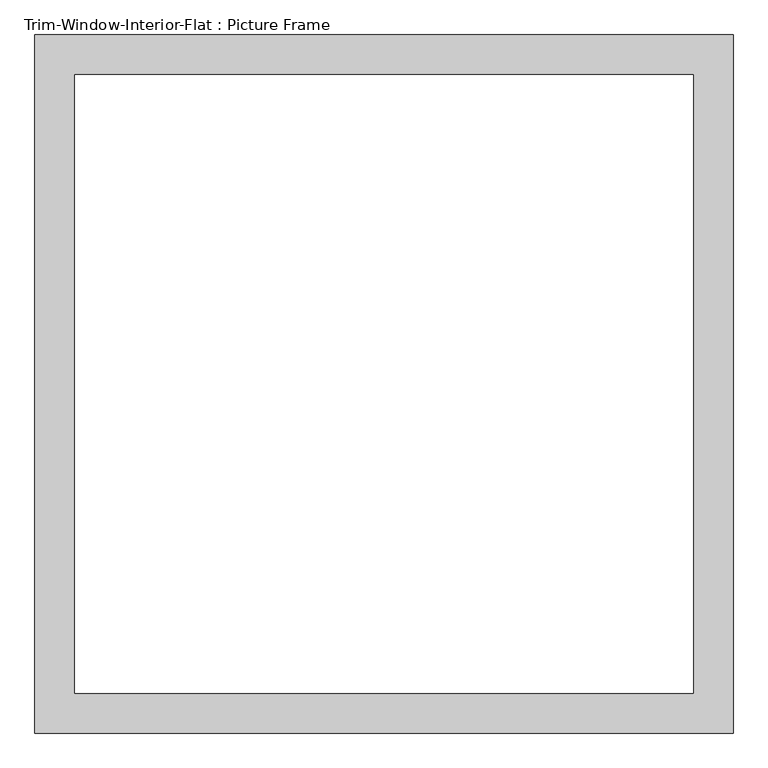
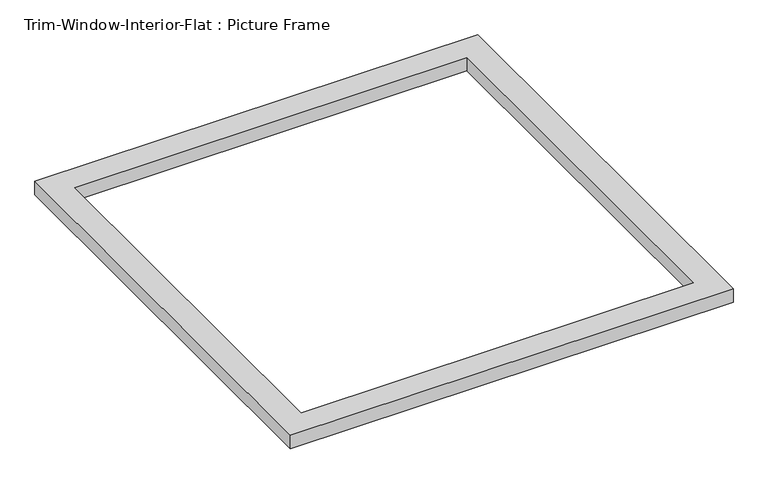
"""IFC4 building model written with IfcOpenShell, lengths in millimetres: proxy geometry, Trim-Window-Interior-Flat : Picture Frame."""

from ifc_helpers import new_model, si_unit, origin, origin_with_axes, place, context, project, spatial, polyline, outline, extrude, source, transform, mapped, element, save


def trim_window_interior_flat_picture_frame_28d4e5dc(model_context):
    return source(origin(), model_context, "Body", "SweptSolid", [
        extrude(outline(polyline([(501.65, 44.45), (501.65, -958.85), (-501.65, -958.85), (-501.65, 44.45), (501.65, 44.45)]), holes=[polyline([(444.5, -12.7), (-444.5, -12.7), (-444.5, -901.7), (444.5, -901.7), (444.5, -12.7)])]), origin_with_axes(), (0.0, 0.0, 1.0), 31.75),
    ])


if __name__ == "__main__":
    model = new_model("IFC4")
    model_context = context("Model", 3, world=origin())
    ifc_project = project(units=[si_unit("LENGTHUNIT", "METRE", prefix="MILLI")], contexts=[model_context])
    site = spatial("IfcSite", under=ifc_project)
    building = spatial("IfcBuilding", under=site)
    placement = place(None, origin())
    trim_window_interior_flat_picture_frame_shape = trim_window_interior_flat_picture_frame_28d4e5dc(model_context)
    element("IfcBuildingElementProxy", 1, Name="Trim-Window-Interior-Flat : Picture Frame", ObjectType="Trim-Window-Interior-Flat : Picture Frame", at=placement, inside=building, context=model_context, shape_type="MappedRepresentation", body=[
        mapped(trim_window_interior_flat_picture_frame_shape, transform((0.0, 0.0, 0.0), x_axis=(1.0, 0.0, 0.0), y_axis=(0.0, 1.0, 0.0), z_axis=(0.0, 0.0, 1.0))),
    ])
    save(model, "model.ifc")

# Revit data of these elements
# Type "Trim-Window-Interior-Flat : Picture Frame"
#   Trim Thickness_Picture Frame = 0' - 1 1/4"
#   Trim Width = 0' - 2 1/4"
#   Trim Thickness_with Sill = 0' - 0 3/4"
#   Sill Thickness = 0' - 1 1/4"
#   Opening Width [instance default] = 2' - 0"
#   Opening Height [instance default] = 3' - 0"
#   Default Elevation = 4' - 0"
#   Sill = no
#   Picture Frame = yes
#   Trim Material [instance default] = none
# Element 1 (IfcBuildingElementProxy, "Trim-Window-Interior-Flat : Picture Frame")
#   Opening Width = 3' - 0"
